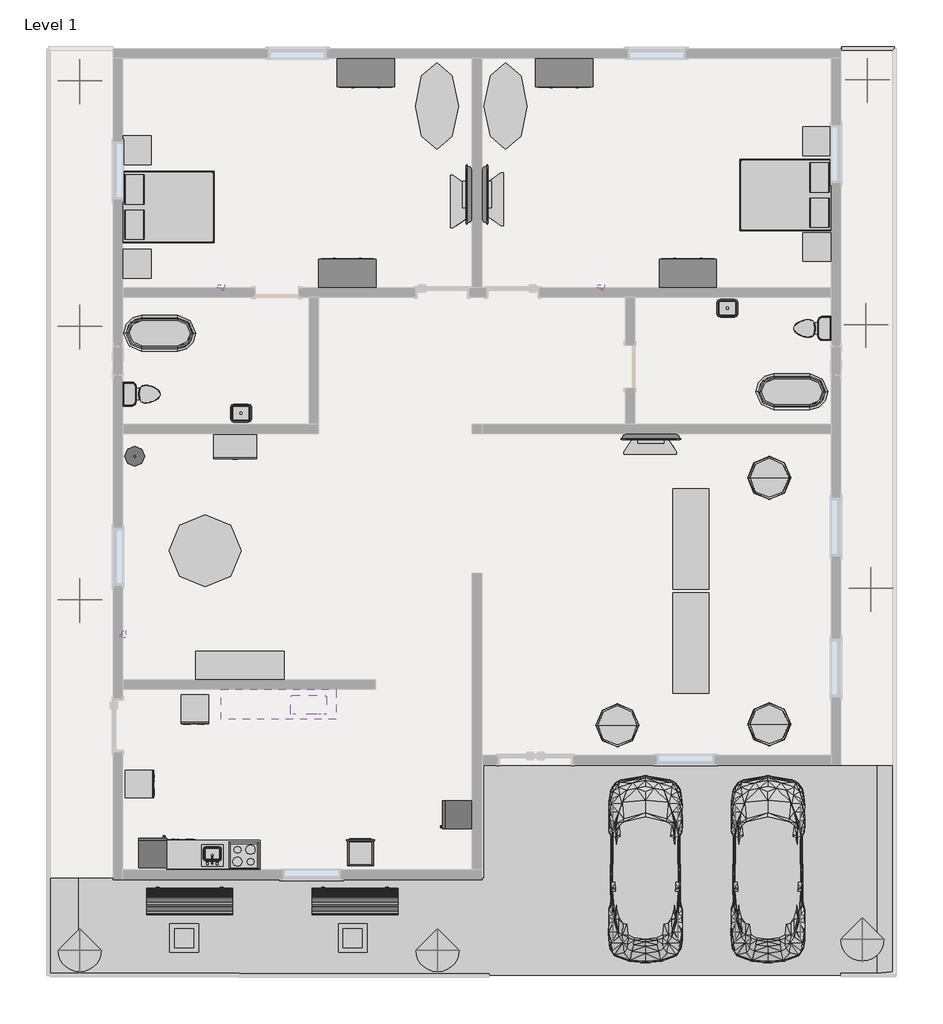
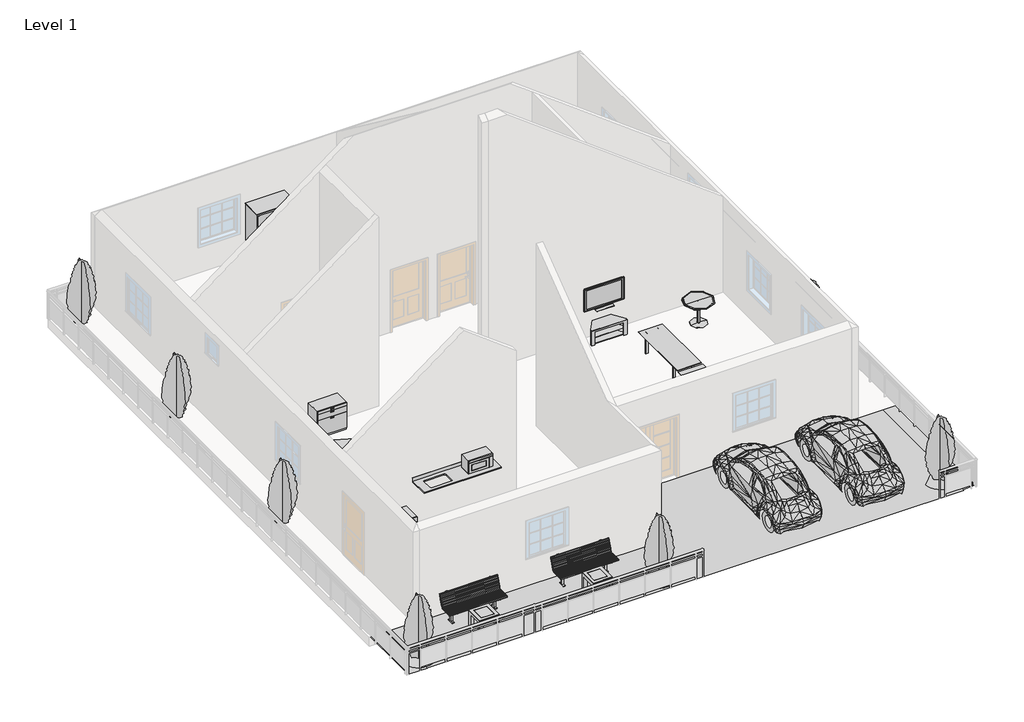
# One storey, part 3 of 3: 30 furniture elements, 17 proxies, 11 geographic elements, 8 flow terminals, 1 railing.
"""IFC4 building model written with IfcOpenShell, lengths in millimetres."""

from ifc_helpers import new_model, si_unit, point, frame, origin, origin_with_axes, place, context, project, spatial, polyline, ellipse_curve, trimmed, outline, extrude, triangles, transform, mapped, element, save
from ifc_brep_helpers import plane_surface, extruded_surface, advanced_brep
from components import proxy_a6faaae8, proxy_53e5fb40, proxy_45b28599, kitchenette_medium_kitchenette_medium_844211aa, proxy_8a8d5ab2, proxy_8b8c2dc4, rpc_beetle_rpc_beetle_3ce7ba48, rpc_picture_frame_rpc_picture_frame_c25e3fe9, proxy_c523a7b7, proxy_66164f77, flow_terminal_871c2e40, flow_terminal_d49f872f, flow_terminal_62a433f7, toilet_domestic_3d_toilet_domestic_3d_f7549cf7, toilet_domestic_3d_toilet_domestic_3d_183bbd19, flow_terminal_b374fae2, furniture_1d2926bd, furniture_c6510c7c, counter_top_w_sink_hole_counter_top_w_sink_hole_22cae41e, furniture_7b927048, furniture_9fa109b2, furniture_e1dba61b, furniture_fdf74506, tv_stand_tv_stand_6ce107e5, furniture_b5c51a22, furniture_92191dda, furniture_bbcc68ce, furniture_027a2ad9, furniture_5bc9ed15, furniture_c80d6d9c, geographic_element_235d1464, rpc_tree_conifer_chinese_juniper_7_1b9786cd

model = new_model("IFC4")

# Units and contexts
model_context = context("Model", 3, world=origin())
ifc_project = project(units=[si_unit("LENGTHUNIT", "METRE", prefix="MILLI")], contexts=[model_context])

# Site, building, storey
site = spatial("IfcSite", under=ifc_project)
building = spatial("IfcBuilding", under=site)
storey = spatial("IfcBuildingStorey", under=building, Name="Level 1", Elevation=0.0)

# Proxies
placement = place(None, origin())
element("IfcBuildingElementProxy", 1, Name="Building Element Proxy", at=placement, inside=storey, context=model_context, shape_type="Tessellation", body=[
    triangles([(-17842.0888458, 13557.9549957, 0.0), (-17105.9465698, 13557.9549957, 0.0), (-17842.0888458, -6127.0451981, 0.0), (-17080.0888458, -4095.0451012, 0.0), (-9244.1892334, -4095.0451012, 0.0), (-9244.1892334, -1656.6451012, 0.0), (-849.4892818, -1762.0254421, 0.0), (-849.4892818, -6127.0451981, 0.0), (-1611.4892818, 13557.9549957, 0.0), (-849.4892818, 13557.9549957, 0.0)], [[3, 4, 1], [6, 4, 5], [4, 2, 1], [2, 4, 6], [2, 6, 9], [7, 6, 5], [4, 3, 5], [5, 8, 7], [8, 5, 3], [9, 7, 10], [9, 6, 7]], closed=False),
])
element("IfcBuildingElementProxy", 2, Name="Building Element Proxy", at=placement, inside=storey, context=model_context, shape_type="Tessellation", body=[
    triangles([(-17817.3124512, -6127.0451981, 0.0), (-18419.3594238, -6127.0451981, 0.0), (-17816.6892334, 13557.9549957, 0.0), (-18438.989621, 13548.4299957, 0.0)], [[4, 2, 1], [1, 3, 4]], closed=False),
])
element("IfcBuildingElementProxy", 3, Name="Building Element Proxy", at=placement, inside=storey, context=model_context, shape_type="Tessellation", body=[
    triangles([(-851.4358927, -6086.4848831, 0.0), (-443.0892697, -6044.4950043, 0.0), (-490.7142697, 13573.8296082, 0.0), (-849.4892818, 13557.9549957, 0.0)], [[4, 1, 2], [2, 3, 4]], closed=False),
])
proxy_shape = proxy_a6faaae8(model_context)
element("IfcBuildingElementProxy", 4, Name="Cook Top-4 Unit2 : 22\" x 20\"", ObjectType="Cook Top-4 Unit2 : 22\" x 20\"", at=placement, inside=storey, context=model_context, shape_type="MappedRepresentation", body=[
    mapped(proxy_shape, transform((-14298.7892853, -3587.0450825, 0.0), x_axis=(-1.0000000000000004, 0.0, 0.0), y_axis=(0.0, -1.0000000000000004, 0.0), z_axis=(0.0, 0.0, 1.0))),
])
proxy_2_shape = proxy_53e5fb40(model_context)
element("IfcBuildingElementProxy", 5, Name="Dishwasher : 23\" x 23 11/16\" x 33 1/2\"", ObjectType="Dishwasher : 23\" x 23 11/16\" x 33 1/2\"", at=placement, inside=storey, context=model_context, shape_type="MappedRepresentation", body=[
    mapped(proxy_2_shape, transform((-16265.9718168, -2439.5330177, 0.0), x_axis=(0.0, 1.0000000000000009, 0.0), y_axis=(-1.0000000000000009, 0.0, 0.0), z_axis=(0.0, 0.0, 1.0))),
])
element("IfcBuildingElementProxy", 6, Name="Dishwasher : 23\" x 23 11/16\" x 33 1/2\"", ObjectType="Dishwasher : 23\" x 23 11/16\" x 33 1/2\"", at=placement, inside=storey, context=model_context, shape_type="MappedRepresentation", body=[
    mapped(proxy_2_shape, transform((-15711.1242223, -733.806712, 0.0), x_axis=(1.0000000000000002, 0.0, 0.0), y_axis=(0.0, 1.0000000000000002, 0.0), z_axis=(0.0, 0.0, 1.0))),
])
proxy_3_shape = proxy_45b28599(model_context)
element("IfcBuildingElementProxy", 7, Name="Dishwasher : 24\" x 24\" x 34\"", ObjectType="Dishwasher : 24\" x 24\" x 34\"", at=placement, inside=storey, context=model_context, shape_type="MappedRepresentation", body=[
    mapped(proxy_3_shape, transform((-15249.9718168, -3295.1955177, 0.0), x_axis=(-1.0000000000000004, 0.0, 0.0), y_axis=(0.0, -1.0000000000000004, 0.0), z_axis=(0.0, 0.0, 1.0))),
])
kitchenette_medium_kitchenette_medium_shape = kitchenette_medium_kitchenette_medium_844211aa(model_context)
element("IfcBuildingElementProxy", 8, Name="Kitchenette - Medium : Kitchenette - Medium", ObjectType="Kitchenette - Medium : Kitchenette - Medium", at=placement, inside=storey, context=model_context, shape_type="MappedRepresentation", body=[
    mapped(kitchenette_medium_kitchenette_medium_shape, transform((-14622.9515804, -3891.8450825, 0.0), x_axis=(-1.0000000000000004, 0.0, 0.0), y_axis=(0.0, -1.0000000000000004, 0.0), z_axis=(0.0, 0.0, 1.0))),
])
proxy_4_shape = proxy_8a8d5ab2(model_context)
element("IfcBuildingElementProxy", 9, Name="Microwave : 30\" x 16\" x 18\"", ObjectType="Microwave : 30\" x 16\" x 18\"", at=placement, inside=storey, context=model_context, shape_type="MappedRepresentation", body=[
    mapped(proxy_4_shape, transform((-13427.4821626, -27.2145766, 609.6), x_axis=(1.0, 0.0, 0.0), y_axis=(0.0, 1.0, 0.0), z_axis=(0.0, 0.0, 1.0))),
])
proxy_5_shape = proxy_8b8c2dc4(model_context)
element("IfcBuildingElementProxy", 10, Name="Oven Double-Built-in : 21 1/2\" x 39 1/4\" x 21\"", ObjectType="Oven Double-Built-in : 21 1/2\" x 39 1/4\" x 21\"", at=placement, inside=storey, context=model_context, shape_type="MappedRepresentation", body=[
    mapped(proxy_5_shape, transform((-11857.4642126, -3395.1792235, 0.0), x_axis=(-1.0000000000000013, 0.0, 0.0), y_axis=(0.0, -1.0000000000000013, 0.0), z_axis=(0.0, 0.0, 1.0))),
])
rpc_beetle_rpc_beetle_shape = rpc_beetle_rpc_beetle_3ce7ba48(model_context)
element("IfcBuildingElementProxy", 11, Name="RPC Beetle : RPC Beetle", ObjectType="RPC Beetle : RPC Beetle", at=placement, inside=storey, context=model_context, shape_type="MappedRepresentation", body=[
    mapped(rpc_beetle_rpc_beetle_shape, transform((-3160.8892853, -5111.0450825, 0.0), x_axis=(1.0, 0.0, 0.0), y_axis=(0.0, 1.0, 0.0), z_axis=(0.0, 0.0, 1.0))),
])
element("IfcBuildingElementProxy", 12, Name="RPC Beetle : RPC Beetle", ObjectType="RPC Beetle : RPC Beetle", at=placement, inside=storey, context=model_context, shape_type="MappedRepresentation", body=[
    mapped(rpc_beetle_rpc_beetle_shape, transform((-5764.3892853, -5111.0450825, 0.0), x_axis=(1.0, 0.0, 0.0), y_axis=(0.0, 1.0, 0.0), z_axis=(0.0, 0.0, 1.0))),
])
rpc_picture_frame_rpc_picture_frame_shape = rpc_picture_frame_rpc_picture_frame_c25e3fe9(model_context)
element("IfcBuildingElementProxy", 13, Name="RPC Picture Frame : RPC Picture Frame", ObjectType="RPC Picture Frame : RPC Picture Frame", at=placement, inside=storey, context=model_context, shape_type="MappedRepresentation", body=[
    mapped(rpc_picture_frame_rpc_picture_frame_shape, transform((-14782.9146553, 8477.9549175, 2133.6), x_axis=(-1.0000000000000004, 0.0, 0.0), y_axis=(0.0, -1.0000000000000004, 0.0), z_axis=(0.0, 0.0, 1.0))),
])
element("IfcBuildingElementProxy", 14, Name="RPC Picture Frame : RPC Picture Frame", ObjectType="RPC Picture Frame : RPC Picture Frame", at=placement, inside=storey, context=model_context, shape_type="MappedRepresentation", body=[
    mapped(rpc_picture_frame_rpc_picture_frame_shape, transform((-6713.5023261, 8477.9549175, 2133.6), x_axis=(-1.0, 0.0, 0.0), y_axis=(0.0, -1.0, 0.0), z_axis=(0.0, 0.0, 1.0))),
])
element("IfcBuildingElementProxy", 15, Name="RPC Picture Frame : RPC Picture Frame", ObjectType="RPC Picture Frame : RPC Picture Frame", at=placement, inside=storey, context=model_context, shape_type="MappedRepresentation", body=[
    mapped(rpc_picture_frame_rpc_picture_frame_shape, transform((-16876.8892853, 1119.0822446, 2133.6), x_axis=(0.0, 1.0000000000000004, 0.0), y_axis=(-1.0000000000000004, 0.0, 0.0), z_axis=(0.0, 0.0, 1.0))),
])
proxy_6_shape = proxy_c523a7b7(model_context)
element("IfcBuildingElementProxy", 16, Name="Refrigerator : 24\" x 25\" LH", ObjectType="Refrigerator : 24\" x 25\" LH", at=placement, inside=storey, context=model_context, shape_type="MappedRepresentation", body=[
    mapped(proxy_6_shape, transform((-16235.5392853, -3541.396111, 0.0), x_axis=(-1.0000000000000004, 0.0, 0.0), y_axis=(0.0, -1.0000000000000004, 0.0), z_axis=(0.0, 0.0, 1.0))),
])
proxy_7_shape = proxy_66164f77(model_context)
element("IfcBuildingElementProxy", 17, Name="Refrigerator : 24\" x 25\" RH", ObjectType="Refrigerator : 24\" x 25\" RH", at=placement, inside=storey, context=model_context, shape_type="MappedRepresentation", body=[
    mapped(proxy_7_shape, transform((-9745.8392853, -2718.2940539, 0.0), x_axis=(0.0, -1.0000000000000007, 0.0), y_axis=(1.0000000000000007, 0.0, 0.0), z_axis=(0.0, 0.0, 1.0))),
])

# Flow terminals
flow_terminal_shape = flow_terminal_871c2e40(model_context)
element("IfcFlowTerminal", 18, ObjectType="Sink Kitchen-Island : 18\" x 18\"", at=placement, inside=storey, context=model_context, shape_type="MappedRepresentation", body=[
    mapped(flow_terminal_shape, transform((-14956.2000447, -3584.6996813, -14.4), x_axis=(-1.0000000000000004, 0.0, 0.0), y_axis=(0.0, -1.0000000000000004, 0.0), z_axis=(0.0, 0.0, 1.0))),
])
flow_terminal_2_shape = flow_terminal_d49f872f(model_context)
element("IfcFlowTerminal", 19, ObjectType="Sink Vanity-Round : 19\" x 19\"", at=placement, inside=storey, context=model_context, shape_type="MappedRepresentation", body=[
    mapped(flow_terminal_2_shape, transform((-16533.4036272, 4799.903177, 609.6), x_axis=(0.0, 1.0, 0.0), y_axis=(-1.0, 0.0, 0.0), z_axis=(0.0, 0.0, 1.0))),
])
flow_terminal_3_shape = flow_terminal_62a433f7(model_context)
element("IfcFlowTerminal", 20, ObjectType="Sink Vanity-Square : 20\" x 18\"", at=placement, inside=storey, context=model_context, shape_type="MappedRepresentation", body=[
    mapped(flow_terminal_3_shape, transform((-14346.6000447, 5762.5003187, 609.6), x_axis=(-1.0000000000000004, 0.0, 0.0), y_axis=(0.0, -1.0000000000000004, 0.0), z_axis=(0.0, 0.0, 1.0))),
])
element("IfcFlowTerminal", 21, ObjectType="Sink Vanity-Square : 20\" x 18\"", at=placement, inside=storey, context=model_context, shape_type="MappedRepresentation", body=[
    mapped(flow_terminal_3_shape, transform((-4040.1785259, 8094.6095164, 609.6), x_axis=(1.0, 0.0, 0.0), y_axis=(0.0, 1.0, 0.0), z_axis=(0.0, 0.0, 1.0))),
])
toilet_domestic_3d_toilet_domestic_3d_shape = toilet_domestic_3d_toilet_domestic_3d_f7549cf7(model_context)
toilet_domestic_3d_toilet_domestic_3d_2_shape = toilet_domestic_3d_toilet_domestic_3d_183bbd19(model_context)
element("IfcFlowTerminal", 22, ObjectType="Toilet-Domestic-3D : Toilet-Domestic-3D", at=placement, inside=storey, context=model_context, shape_type="MappedRepresentation", body=[
    mapped(toilet_domestic_3d_toilet_domestic_3d_shape, transform((-2309.3853126, 7614.3549175, 0.0), x_axis=(0.0, -1.0, 0.0), y_axis=(1.0, 0.0, 0.0), z_axis=(0.0, 0.0, 1.0))),
    mapped(toilet_domestic_3d_toilet_domestic_3d_2_shape, transform((-2309.3853126, 7614.3549175, 0.0), x_axis=(0.0, -1.0, 0.0), y_axis=(1.0, 0.0, 0.0), z_axis=(0.0, 0.0, 1.0))),
])
element("IfcFlowTerminal", 23, ObjectType="Toilet-Domestic-3D : Toilet-Domestic-3D", at=placement, inside=storey, context=model_context, shape_type="MappedRepresentation", body=[
    mapped(toilet_domestic_3d_toilet_domestic_3d_shape, transform((-16382.1932579, 6217.3549175, 0.0), x_axis=(0.0, 1.0000000000000002, 0.0), y_axis=(-1.0000000000000002, 0.0, 0.0), z_axis=(0.0, 0.0, 1.0))),
    mapped(toilet_domestic_3d_toilet_domestic_3d_2_shape, transform((-16382.1932579, 6217.3549175, 0.0), x_axis=(0.0, 1.0000000000000002, 0.0), y_axis=(-1.0000000000000002, 0.0, 0.0), z_axis=(0.0, 0.0, 1.0))),
])
flow_terminal_4_shape = flow_terminal_b374fae2(model_context)
element("IfcFlowTerminal", 24, ObjectType="Tub-Free Standing-3D : 30\" x 60\"", at=placement, inside=storey, context=model_context, shape_type="MappedRepresentation", body=[
    mapped(flow_terminal_4_shape, transform((-16089.4892853, 7512.7549175, 0.0), x_axis=(0.0, 1.0000000000000002, 0.0), y_axis=(-1.0000000000000002, 0.0, 0.0), z_axis=(0.0, 0.0, 1.0))),
])
element("IfcFlowTerminal", 25, ObjectType="Tub-Free Standing-3D : 30\" x 60\"", at=placement, inside=storey, context=model_context, shape_type="MappedRepresentation", body=[
    mapped(flow_terminal_4_shape, transform((-2652.8892853, 6268.1549175, 0.0), x_axis=(0.0, -1.0000000000000009, 0.0), y_axis=(1.0000000000000009, 0.0, 0.0), z_axis=(0.0, 0.0, 1.0))),
])

# Furniture
furniture_shape = furniture_1d2926bd(model_context)
element("IfcFurniture", 26, ObjectType="Bed-Box : Queen 60\" x 79\"", at=placement, inside=storey, context=model_context, shape_type="MappedRepresentation", body=[
    mapped(furniture_shape, transform((-16171.5187935, 9853.3024585, 0.0), x_axis=(0.0, 1.0000000000000002, 0.0), y_axis=(-1.0000000000000002, 0.0, 0.0), z_axis=(0.0, 0.0, 1.0))),
])
element("IfcFurniture", 27, ObjectType="Bed-Box : Queen 60\" x 79\"", at=placement, inside=storey, context=model_context, shape_type="MappedRepresentation", body=[
    mapped(furniture_shape, transform((-2520.0597771, 10785.6073766, 0.0), x_axis=(0.0, -1.0000000000000004, 0.0), y_axis=(1.0000000000000004, 0.0, 0.0), z_axis=(0.0, 0.0, 1.0))),
])
furniture_2_shape = furniture_c6510c7c(model_context)
element("IfcFurniture", 28, ObjectType="Counter Top w Sink Hole : 24\" Depth", at=placement, inside=storey, context=model_context, shape_type="MappedRepresentation", body=[
    mapped(furniture_2_shape, transform((-15156.3515804, -3891.8450825, -14.4), x_axis=(-1.0000000000000004, 0.0, 0.0), y_axis=(0.0, -1.0000000000000004, 0.0), z_axis=(0.0, 0.0, 1.0))),
])
counter_top_w_sink_hole_counter_top_w_sink_hole_shape = counter_top_w_sink_hole_counter_top_w_sink_hole_22cae41e(model_context)
element("IfcFurniture", 29, ObjectType="Counter Top w Sink Hole : Counter Top w Sink Hole", at=placement, inside=storey, context=model_context, shape_type="MappedRepresentation", body=[
    mapped(counter_top_w_sink_hole_counter_top_w_sink_hole_shape, transform((-13580.9269902, -56.4450825, 609.6), x_axis=(1.0, 0.0, 0.0), y_axis=(0.0, 1.0, 0.0), z_axis=(0.0, 0.0, 1.0))),
])
furniture_3_shape = furniture_7b927048(model_context)
element("IfcFurniture", 30, ObjectType="Credenza : 72\" x 24\"", at=placement, inside=storey, context=model_context, shape_type="MappedRepresentation", body=[
    mapped(furniture_3_shape, transform((-14447.2335476, 446.9745897, 0.0), x_axis=(1.0, 0.0, 0.0), y_axis=(0.0, 1.0, 0.0), z_axis=(0.0, 0.0, 1.0))),
])
furniture_4_shape = furniture_9fa109b2(model_context)
element("IfcFurniture", 31, ObjectType="Dresser : 48\" x 72\" x 24\"", at=placement, inside=storey, context=model_context, shape_type="MappedRepresentation", body=[
    mapped(furniture_4_shape, transform((-12370.8825451, 8419.5919634, 0.0), x_axis=(-1.0000000000000004, 0.0, 0.0), y_axis=(0.0, -1.0000000000000004, 0.0), z_axis=(0.0, 0.0, 1.0))),
])
element("IfcFurniture", 32, ObjectType="Dresser : 48\" x 72\" x 24\"", at=placement, inside=storey, context=model_context, shape_type="MappedRepresentation", body=[
    mapped(furniture_4_shape, transform((-11438.7960255, 13413.1178716, 0.0), x_axis=(1.0, 0.0, 0.0), y_axis=(0.0, 1.0, 0.0), z_axis=(0.0, 0.0, 1.0))),
])
element("IfcFurniture", 33, ObjectType="Dresser : 48\" x 72\" x 24\"", at=placement, inside=storey, context=model_context, shape_type="MappedRepresentation", body=[
    mapped(furniture_4_shape, transform((-7222.3960255, 13413.1178716, 0.0), x_axis=(1.0, 0.0, 0.0), y_axis=(0.0, 1.0, 0.0), z_axis=(0.0, 0.0, 1.0))),
])
element("IfcFurniture", 34, ObjectType="Dresser : 48\" x 72\" x 24\"", at=placement, inside=storey, context=model_context, shape_type="MappedRepresentation", body=[
    mapped(furniture_4_shape, transform((-5131.8825451, 8419.5919634, 0.0), x_axis=(-1.0000000000000004, 0.0, 0.0), y_axis=(0.0, -1.0000000000000004, 0.0), z_axis=(0.0, 0.0, 1.0))),
])
furniture_5_shape = furniture_e1dba61b(model_context)
element("IfcFurniture", 35, ObjectType="Storage Pedestal : 20\" x 36\" x 36\"", at=placement, inside=storey, context=model_context, shape_type="MappedRepresentation", body=[
    mapped(furniture_5_shape, transform((-14309.2667714, 6034.0732936, 0.0), x_axis=(1.0, 0.0, 0.0), y_axis=(0.0, 1.0, 0.0), z_axis=(0.0, 0.0, 1.0))),
])
furniture_6_shape = furniture_fdf74506(model_context)
element("IfcFurniture", 36, ObjectType="TV - Flat Screen : 50\"", at=placement, inside=storey, context=model_context, shape_type="MappedRepresentation", body=[
    mapped(furniture_6_shape, transform((-9505.9279089, 10455.2104034, 914.4), x_axis=(0.0, -1.0000000000000004, 0.0), y_axis=(1.0000000000000004, 0.0, 0.0), z_axis=(0.0, 0.0, 1.0))),
])
element("IfcFurniture", 37, ObjectType="TV - Flat Screen : 50\"", at=placement, inside=storey, context=model_context, shape_type="MappedRepresentation", body=[
    mapped(furniture_6_shape, transform((-9185.6506616, 10463.0994317, 914.4), x_axis=(0.0, 1.0000000000000002, 0.0), y_axis=(-1.0000000000000002, 0.0, 0.0), z_axis=(0.0, 0.0, 1.0))),
])
element("IfcFurniture", 38, ObjectType="TV - Flat Screen : 50\"", at=placement, inside=storey, context=model_context, shape_type="MappedRepresentation", body=[
    mapped(furniture_6_shape, transform((-5646.1447711, 5320.6162939, 914.4), x_axis=(1.0, 0.0, 0.0), y_axis=(0.0, 1.0, 0.0), z_axis=(0.0, 0.0, 1.0))),
])
tv_stand_tv_stand_shape = tv_stand_tv_stand_6ce107e5(model_context)
element("IfcFurniture", 39, ObjectType="TV Stand : TV Stand", at=placement, inside=storey, context=model_context, shape_type="MappedRepresentation", body=[
    mapped(tv_stand_tv_stand_shape, transform((-9447.3892853, 10431.9429196, 0.0), x_axis=(0.0, -1.0, 0.0), y_axis=(1.0, 0.0, 0.0), z_axis=(0.0, 0.0, 1.0))),
])
element("IfcFurniture", 40, ObjectType="TV Stand : TV Stand", at=placement, inside=storey, context=model_context, shape_type="MappedRepresentation", body=[
    mapped(tv_stand_tv_stand_shape, transform((-9244.1892853, 10232.3669155, 0.0), x_axis=(0.0, 1.0, 0.0), y_axis=(-1.0, 0.0, 0.0), z_axis=(0.0, 0.0, 1.0))),
])
element("IfcFurniture", 41, ObjectType="TV Stand : TV Stand", at=placement, inside=storey, context=model_context, shape_type="MappedRepresentation", body=[
    mapped(tv_stand_tv_stand_shape, transform((-5787.4891902, 5402.9061632, 0.0), x_axis=(1.0000000000000007, 0.0, 0.0), y_axis=(0.0, 1.0000000000000007, 0.0), z_axis=(0.0, 0.0, 1.0))),
])
furniture_7_shape = furniture_b5c51a22(model_context)
element("IfcFurniture", 42, ObjectType="Table-Coffee : 24\" x 24\" x 24\"", at=placement, inside=storey, context=model_context, shape_type="MappedRepresentation", body=[
    mapped(furniture_7_shape, transform((-15587.055052, -5434.8561603, 0.0), x_axis=(1.0, 0.0, 0.0), y_axis=(0.0, 1.0, 0.0), z_axis=(0.0, 0.0, 1.0))),
])
element("IfcFurniture", 43, ObjectType="Table-Coffee : 24\" x 24\" x 24\"", at=placement, inside=storey, context=model_context, shape_type="MappedRepresentation", body=[
    mapped(furniture_7_shape, transform((-12005.655052, -5434.8561603, 0.0), x_axis=(1.0, 0.0, 0.0), y_axis=(0.0, 1.0, 0.0), z_axis=(0.0, 0.0, 1.0))),
])
furniture_8_shape = furniture_92191dda(model_context)
element("IfcFurniture", 44, ObjectType="Table-Dining : 30\" x 84\" x 22\"", at=placement, inside=storey, context=model_context, shape_type="MappedRepresentation", body=[
    mapped(furniture_8_shape, transform((-4703.9782075, 915.8891509, 0.0), x_axis=(0.0, 1.0, 0.0), y_axis=(-1.0, 0.0, 0.0), z_axis=(0.0, 0.0, 1.0))),
])
element("IfcFurniture", 45, ObjectType="Table-Dining : 30\" x 84\" x 22\"", at=placement, inside=storey, context=model_context, shape_type="MappedRepresentation", body=[
    mapped(furniture_8_shape, transform((-4703.9782075, 3125.6891509, 0.0), x_axis=(0.0, 1.0, 0.0), y_axis=(-1.0, 0.0, 0.0), z_axis=(0.0, 0.0, 1.0))),
])
furniture_9_shape = furniture_bbcc68ce(model_context)
element("IfcFurniture", 46, ObjectType="Table-Dining Round w Chairs : 60\" Diameter", at=placement, inside=storey, context=model_context, shape_type="MappedRepresentation", body=[
    mapped(furniture_9_shape, transform((-15227.9712525, 3074.8336061, 0.0), x_axis=(1.0, 0.0, 0.0), y_axis=(0.0, 1.0, 0.0), z_axis=(0.0, 0.0, 1.0))),
])
furniture_10_shape = furniture_027a2ad9(model_context)
element("IfcFurniture", 47, ObjectType="Table-Ellipse : 72\" x 36\"", at=placement, inside=storey, context=model_context, shape_type="MappedRepresentation", body=[
    mapped(furniture_10_shape, transform((-8736.1892853, 12338.7549175, 0.0), x_axis=(0.0, 1.0000000000000002, 0.0), y_axis=(-1.0000000000000002, 0.0, 0.0), z_axis=(0.0, 0.0, 1.0))),
])
element("IfcFurniture", 48, ObjectType="Table-Ellipse : 72\" x 36\"", at=placement, inside=storey, context=model_context, shape_type="MappedRepresentation", body=[
    mapped(furniture_10_shape, transform((-10196.6892853, 12338.7549175, 0.0), x_axis=(0.0, 1.0000000000000002, 0.0), y_axis=(-1.0000000000000002, 0.0, 0.0), z_axis=(0.0, 0.0, 1.0))),
])
furniture_11_shape = furniture_5bc9ed15(model_context)
element("IfcFurniture", 49, ObjectType="Table-Night Stand : 24\" x 24\" x 30\"", at=placement, inside=storey, context=model_context, shape_type="MappedRepresentation", body=[
    mapped(furniture_11_shape, transform((-16880.6229156, 8681.1549175, 0.0), x_axis=(1.0, 0.0, 0.0), y_axis=(0.0, 1.0, 0.0), z_axis=(0.0, 0.0, 1.0))),
])
element("IfcFurniture", 50, ObjectType="Table-Night Stand : 24\" x 24\" x 30\"", at=placement, inside=storey, context=model_context, shape_type="MappedRepresentation", body=[
    mapped(furniture_11_shape, transform((-16880.6229156, 11094.1549175, 0.0), x_axis=(1.0, 0.0, 0.0), y_axis=(0.0, 1.0, 0.0), z_axis=(0.0, 0.0, 1.0))),
])
element("IfcFurniture", 51, ObjectType="Table-Night Stand : 24\" x 24\" x 30\"", at=placement, inside=storey, context=model_context, shape_type="MappedRepresentation", body=[
    mapped(furniture_11_shape, transform((-2428.0229156, 9036.7549175, 0.0), x_axis=(1.0, 0.0, 0.0), y_axis=(0.0, 1.0, 0.0), z_axis=(0.0, 0.0, 1.0))),
])
element("IfcFurniture", 52, ObjectType="Table-Night Stand : 24\" x 24\" x 30\"", at=placement, inside=storey, context=model_context, shape_type="MappedRepresentation", body=[
    mapped(furniture_11_shape, transform((-2428.0229156, 11284.6549175, 0.0), x_axis=(1.0, 0.0, 0.0), y_axis=(0.0, 1.0, 0.0), z_axis=(0.0, 0.0, 1.0))),
])
furniture_12_shape = furniture_c80d6d9c(model_context)
element("IfcFurniture", 53, ObjectType="Table-Round : 36\" Diameter", at=placement, inside=storey, context=model_context, shape_type="MappedRepresentation", body=[
    mapped(furniture_12_shape, transform((-3135.4892853, -799.3950825, 0.0), x_axis=(1.0, 0.0, 0.0), y_axis=(0.0, 1.0, 0.0), z_axis=(0.0, 0.0, 1.0))),
])
element("IfcFurniture", 54, ObjectType="Table-Round : 36\" Diameter", at=placement, inside=storey, context=model_context, shape_type="MappedRepresentation", body=[
    mapped(furniture_12_shape, transform((-6361.2892853, -818.4450825, 0.0), x_axis=(1.0, 0.0, 0.0), y_axis=(0.0, 1.0, 0.0), z_axis=(0.0, 0.0, 1.0))),
])
element("IfcFurniture", 55, ObjectType="Table-Round : 36\" Diameter", at=placement, inside=storey, context=model_context, shape_type="MappedRepresentation", body=[
    mapped(furniture_12_shape, transform((-3135.4892853, 4439.3549175, 0.0), x_axis=(1.0, 0.0, 0.0), y_axis=(0.0, 1.0, 0.0), z_axis=(0.0, 0.0, 1.0))),
])

# Geographic elements
geographic_element_shape = geographic_element_235d1464(model_context)
element("IfcGeographicElement", 56, ObjectType="Park Bench : 72\"", at=placement, inside=storey, context=model_context, shape_type="MappedRepresentation", body=[
    mapped(geographic_element_shape, transform((-11936.5892853, -4526.8450825, 0.0), x_axis=(1.0, 0.0, 0.0), y_axis=(0.0, 1.0, 0.0), z_axis=(0.0, 0.0, 1.0))),
])
element("IfcGeographicElement", 57, ObjectType="Park Bench : 72\"", at=placement, inside=storey, context=model_context, shape_type="MappedRepresentation", body=[
    mapped(geographic_element_shape, transform((-15454.4892853, -4526.8450825, 0.0), x_axis=(1.0, 0.0, 0.0), y_axis=(0.0, 1.0, 0.0), z_axis=(0.0, 0.0, 1.0))),
])
rpc_tree_conifer_chinese_juniper_7_shape = rpc_tree_conifer_chinese_juniper_7_1b9786cd(model_context)
element("IfcGeographicElement", 58, ObjectType="RPC Tree - Conifer : Chinese Juniper - 7'", at=placement, inside=storey, context=model_context, shape_type="MappedRepresentation", body=[
    mapped(rpc_tree_conifer_chinese_juniper_7_shape, transform((-1154.4859564, -5365.0450825, 0.0), x_axis=(1.0, 0.0, 0.0), y_axis=(0.0, 1.0, 0.0), z_axis=(0.0, 0.0, 1.0))),
])
element("IfcGeographicElement", 59, ObjectType="RPC Tree - Conifer : Chinese Juniper - 7'", at=placement, inside=storey, context=model_context, shape_type="MappedRepresentation", body=[
    mapped(rpc_tree_conifer_chinese_juniper_7_shape, transform((-10184.1859564, -5593.6450825, 0.0), x_axis=(1.0, 0.0, 0.0), y_axis=(0.0, 1.0, 0.0), z_axis=(0.0, 0.0, 1.0))),
])
element("IfcGeographicElement", 60, ObjectType="RPC Tree - Conifer : Chinese Juniper - 7'", at=placement, inside=storey, context=model_context, shape_type="MappedRepresentation", body=[
    mapped(rpc_tree_conifer_chinese_juniper_7_shape, transform((-17791.4859564, -5593.6450825, 0.0), x_axis=(1.0, 0.0, 0.0), y_axis=(0.0, 1.0, 0.0), z_axis=(0.0, 0.0, 1.0))),
])
element("IfcGeographicElement", 61, ObjectType="RPC Tree - Conifer : Chinese Juniper - 7'", at=placement, inside=storey, context=model_context, shape_type="MappedRepresentation", body=[
    mapped(rpc_tree_conifer_chinese_juniper_7_shape, transform((-17791.4859564, 1848.5549175, 0.0), x_axis=(1.0, 0.0, 0.0), y_axis=(0.0, 1.0, 0.0), z_axis=(0.0, 0.0, 1.0))),
])
element("IfcGeographicElement", 62, ObjectType="RPC Tree - Conifer : Chinese Juniper - 7'", at=placement, inside=storey, context=model_context, shape_type="MappedRepresentation", body=[
    mapped(rpc_tree_conifer_chinese_juniper_7_shape, transform((-17791.4859564, 7665.1549175, 0.0), x_axis=(1.0, 0.0, 0.0), y_axis=(0.0, 1.0, 0.0), z_axis=(0.0, 0.0, 1.0))),
])
element("IfcGeographicElement", 63, ObjectType="RPC Tree - Conifer : Chinese Juniper - 7'", at=placement, inside=storey, context=model_context, shape_type="MappedRepresentation", body=[
    mapped(rpc_tree_conifer_chinese_juniper_7_shape, transform((-17791.4859564, 12872.1549175, 0.0), x_axis=(1.0, 0.0, 0.0), y_axis=(0.0, 1.0, 0.0), z_axis=(0.0, 0.0, 1.0))),
])
element("IfcGeographicElement", 64, ObjectType="RPC Tree - Conifer : Chinese Juniper - 7'", at=placement, inside=storey, context=model_context, shape_type="MappedRepresentation", body=[
    mapped(rpc_tree_conifer_chinese_juniper_7_shape, transform((-1052.8859564, 12897.5549175, 0.0), x_axis=(1.0, 0.0, 0.0), y_axis=(0.0, 1.0, 0.0), z_axis=(0.0, 0.0, 1.0))),
])
element("IfcGeographicElement", 65, ObjectType="RPC Tree - Conifer : Chinese Juniper - 7'", at=placement, inside=storey, context=model_context, shape_type="MappedRepresentation", body=[
    mapped(rpc_tree_conifer_chinese_juniper_7_shape, transform((-1078.2859564, 7690.5549175, 0.0), x_axis=(1.0, 0.0, 0.0), y_axis=(0.0, 1.0, 0.0), z_axis=(0.0, 0.0, 1.0))),
])
element("IfcGeographicElement", 66, ObjectType="RPC Tree - Conifer : Chinese Juniper - 7'", at=placement, inside=storey, context=model_context, shape_type="MappedRepresentation", body=[
    mapped(rpc_tree_conifer_chinese_juniper_7_shape, transform((-976.6859564, 2089.8549175, 0.0), x_axis=(1.0, 0.0, 0.0), y_axis=(0.0, 1.0, 0.0), z_axis=(0.0, 0.0, 1.0))),
])

# Railing
element("IfcRailing", 67, ObjectType="Glass Panel - Bottom Fill", at=placement, inside=storey, context=model_context, shape_type="SolidModel", body=[
    advanced_brep(
    [(-478.0142853, 13526.2049175, 914.4), (-478.0142853, 13602.4049175, 914.4), (-1595.6142853, 13526.2049175, 914.4), (-1595.6142853, 13602.4049175, 914.4)],
    [
        (0, 1, ellipse_curve(frame((-478.0142853, 13564.3049175, 914.4), z_axis=(1.0, 0.0, 0.0), x_axis=(0.0, 1.0, 0.0)), 38.1, 28.575)),
        (1, 0, ellipse_curve(frame((-478.0142853, 13564.3049175, 914.4), z_axis=(1.0, 0.0, 0.0), x_axis=(0.0, 1.0, 0.0)), 38.1, 28.575)),
        (2, 3, ellipse_curve(frame((-1595.6142853, 13564.3049175, 914.4), z_axis=(-1.0, 0.0, 0.0), x_axis=(0.0, 1.0, 0.0)), 38.1, 28.575)),
        (3, 2, ellipse_curve(frame((-1595.6142853, 13564.3049175, 914.4), z_axis=(-1.0, 0.0, 0.0), x_axis=(0.0, 1.0, 0.0)), 38.1, 28.575)),
        (0, 2),
        (3, 1),
    ],
    [
        plane_surface(frame((-478.0142853, 13564.3049175, 914.4), z_axis=(1.0, 0.0, 0.0), x_axis=(0.0, -1.0, 0.0))),
        plane_surface(frame((-1595.6142853, 13564.3049175, 914.4), z_axis=(-1.0, 0.0, 0.0), x_axis=(0.0, -1.0, 0.0))),
        extruded_surface(trimmed(ellipse_curve(frame((-1595.6142853, 13564.3049175, 914.4), z_axis=(1.0, 0.0, 0.0), x_axis=(0.0, 1.0, 0.0)), 38.1, 28.575), [point((-1595.6142853, 13526.2049175, 914.4))], [point((-1595.6142853, 13602.4049175, 914.4))], True, "CARTESIAN"), (1117.6, 0.0, 0.0), 1117.6),
        extruded_surface(trimmed(ellipse_curve(frame((-1595.6142853, 13564.3049175, 914.4), z_axis=(1.0, 0.0, 0.0), x_axis=(0.0, 1.0, 0.0)), 38.1, 28.575), [point((-1595.6142853, 13602.4049175, 914.4))], [point((-1595.6142853, 13526.2049175, 914.4))], True, "CARTESIAN"), (1117.6, 0.0, 0.0), 1117.6),
    ],
    [
        (0, [[1, 2]]),
        (1, [[3, 4]]),
        (2, [[-1, 5, -4, 6]]),
        (3, [[-2, -6, -3, -5]]),
    ],
),
    extrude(outline(polyline([(-478.0142853, 13577.0049175), (-478.0142853, 13551.6049175), (-1595.6142853, 13551.6049175), (-1595.6142853, 13577.0049175), (-478.0142853, 13577.0049175)])), frame((0.0, 0.0, 800.1), z_axis=(0.0, 0.0, 1.0), x_axis=(1.0, 0.0, 0.0)), (0.0, 0.0, 1.0), 25.4),
    extrude(outline(polyline([(-478.0142853, 13577.0049175), (-478.0142853, 13551.6049175), (-1595.6142853, 13551.6049175), (-1595.6142853, 13577.0049175), (-478.0142853, 13577.0049175)])), frame((0.0, 0.0, 698.5), z_axis=(0.0, 0.0, 1.0), x_axis=(1.0, 0.0, 0.0)), (0.0, 0.0, 1.0), 25.4),
    extrude(outline(polyline([(-1436.8642853, 13589.7049175), (-1436.8642853, 13538.9049175), (-1449.5642853, 13538.9049175), (-1449.5642853, 13589.7049175), (-1436.8642853, 13589.7049175)])), origin_with_axes(), (0.0, 0.0, 1.0), 885.6788223),
    extrude(outline(polyline([(-630.4142853, 13557.7697605), (-1443.2142853, 13557.7697605), (-1443.2142853, 13564.1197605), (-630.4142853, 13564.1197605), (-630.4142853, 13557.7697605)])), frame((0.0, 0.0, 101.6), z_axis=(0.0, 0.0, 1.0), x_axis=(1.0, 0.0, 0.0)), (0.0, 0.0, 1.0), 596.9),
    extrude(outline(polyline([(-624.0642853, 13589.7049175), (-624.0642853, 13538.9049175), (-636.7642853, 13538.9049175), (-636.7642853, 13589.7049175), (-624.0642853, 13589.7049175)])), origin_with_axes(), (0.0, 0.0, 1.0), 885.6788223),
    extrude(outline(polyline([(-1582.9142853, 13573.8299175), (-1582.9142853, 13554.7799175), (-1601.9642853, 13554.7799175), (-1601.9642853, 13573.8299175), (-1582.9142853, 13573.8299175)])), origin_with_axes(), (0.0, 0.0, 1.0), 885.6788223),
    extrude(outline(polyline([(-471.6642853, 13573.8299175), (-471.6642853, 13554.7799175), (-490.7142853, 13554.7799175), (-490.7142853, 13573.8299175), (-471.6642853, 13573.8299175)])), origin_with_axes(), (0.0, 0.0, 1.0), 885.6788223),
])

save(model, "model.ifc")

# Revit data of these elements
# Type "Cook Top-4 Unit2 : 22\" x 20\""
#   Depth = 1' - 8"
#   Width = 1' - 10"
#   Burner Material = Steel, Chrome Plated
#   Cooktop Material = Steel, Polished
#   Default Elevation = 0
#   Assembly Code = ""
# Type "Dishwasher : 23\" x 23 11/16\" x 33 1/2\""
#   Label = "DW"
#   Assembly Code = "E1090400"
#   Depth = 1' - 11 11/16"
#   Height = 2' - 9 1/2"
#   Width = 1' - 11"
#   Dishwasher Material = Steel, Paint Finish, Ivory, Glossy
#   Panel Face Material = Plastic, Opaque Black
#   Default Elevation = 0
# Type "Dishwasher : 24\" x 24\" x 34\""
#   Label = "DW"
#   Assembly Code = "E1090400"
#   Depth = 2' - 0"
#   Height = 2' - 10"
#   Width = 2' - 0"
#   Dishwasher Material = Steel, Paint Finish, Ivory, Glossy
#   Panel Face Material = Plastic, Opaque Black
#   Default Elevation = 0
# Type "Kitchenette - Medium : Kitchenette - Medium"
#   Assembly Code = "E1090400"
#   Counter Length = 6' - 6"
#   Cabinet Width = 4' - 6"
#   Cabinet Height = 2' - 10 1/2"
#   Cabinet Depth = 2' - 0"
#   Toe Depth = 0' - 3"
#   Toe Height = 0' - 3 1/2"
#   Cabinet Material = Cabinets
#   Door/Drawer Material = Cabinets
#   Handle Material = Cabinets - Handles
#   Default Elevation = 0
# Type "Microwave : 30\" x 16\" x 18\""
#   Assembly Code = "E1090400"
#   Depth = 1' - 4"
#   Height = 1' - 6"
#   Width = 2' - 6"
#   Microwave Material = Laminate, Ivory, Matte
#   Default Elevation = 0
# Type "Oven Double-Built-in : 21 1/2\" x 39 1/4\" x 21\""
#   Label = "OVEN"
#   Assembly Code = "E1090400"
#   Depth = 1' - 9"
#   Height = 3' - 3 1/4"
#   Width = 1' - 9 1/2"
#   Oven Material = Metal - Stainless Steel, Polished
#   Default Elevation = 0
# Type "RPC Beetle : RPC Beetle"
#   built-in parameter 1005195 = "RPC-16-0U6E-L4EG-ENH1-J3KF-SVEL-0TX4-C0"
#   Height = 0
# Type "RPC Picture Frame : RPC Picture Frame"
#   built-in parameter 1005198 = "{2, 15},{39, RPC-16-8M5E-0H3T-F0AH-3U0K-JLQ7-G28B-AU},{1, 0},{1, 0},{2, 19},{1, 8},{5, Color},{1, 0},{1, 0},{3, 0.8},{3, 0.8},{3, 0.8},{1, 8},{7, BBoxMin},{1, 0},{1, 0},{1, 0},{1, 0},{1, 0},{1, 8},{7, BBoxMax},{1, 0},{1, 0},{1, 0},{1, 0},{1, 0},{2, 11},{9, RPCTypeId},{1, 0},{1, 0},{39, RPC-16-8M5E-0H3T-F0AH-3U0K-JLQ7-G28B-AU},{1, 6},{14, RPCPlantHeight},{1, 0},{1, 0},{5, 0.625},{2, 11},{7, keyword},{1, 0},{1, 0},{33, :RPCs:Office Clutter:Geometry:RPC},{2, 11},{8, category},{1, 0},{1, 0},{14, Office Clutter},{2, 11},{12, LocalizedUID},{1, 0},{1, 0},{13, Picture Frame},{2, 14},{6, Height},{1, 0},{1, 0},{5, 0.625},{1, 2},{16, Cast Reflections},{1, 0},{1, 0},{1, 0},{1, 2},{8, Portrait},{1, 0},{1, 0},{1, 1},{1, 2},{5, Stand},{1, 0},{1, 0},{1, 1},{2, 11},{10, RPCL_Frame},{1, 0},{1, 0},{5, Frame},{1, 4},{14, Frame Material},{1, 0},{1, 0},{1, 0},{2, 11},{12, RPCL_Picture},{1, 0},{1, 0},{7, Picture},{2, 11},{15, Picture Preview},{1, 0},{1, 0},{65, __RPC:/object data/textures/object/Photo/Photo0/textures/Portrait},{2, 11},{17, i_Picture Preview},{1, 0},{1, 0},{0, },{1, 2},{18, Use Custom Picture},{1, 0},{1, 0},{1, 0},{2, 11},{17, Picture File Name},{1, 0},{1, 0},{0, },{21, assetlibrary_base.fbx},{1, 5},"
#   built-in parameter 1005195 = "RPC-16-8M5E-0H3T-F0AH-3U0K-JLQ7-G28B-AU"
#   Height = 0
# Type "Refrigerator : 24\" x 25\" LH"
#   Label = "REF."
#   Assembly Code = "E1090400"
#   Depth = 2' - 0 3/4"
#   Handle = 0' - 1 1/2"
#   Height = 5' - 3 1/2"
#   Rear Clearance = 0' - 2"
#   Top Door Height = 1' - 8"
#   Width = 1' - 11 1/2"
#   Material = Steel, Paint Finish, Ivory, Glossy
#   Default Elevation = 0
# Type "Refrigerator : 24\" x 25\" RH"
#   Label = "REF."
#   Assembly Code = "E1090400"
#   Depth = 2' - 0 3/4"
#   Handle = 1' - 9"
#   Height = 5' - 3 1/2"
#   Rear Clearance = 0' - 2"
#   Top Door Height = 1' - 8"
#   Width = 1' - 11 1/2"
#   Material = Steel, Paint Finish, Ivory, Glossy
#   Default Elevation = 0
# Type "Sink Kitchen-Island : 18\" x 18\""
#   Assembly Code = "D2010410"
#   Counter Height = 3' - 0"
#   Depth = 1' - 6"
#   Width = 1' - 6"
#   Faucet Material = Steel, Polished
#   Sink Material = Steel, Polished
#   Default Elevation = 0
# Type "Sink Vanity-Round : 19\" x 19\""
#   Assembly Code = "D2010400"
#   Top Of Counter = 2' - 7"
#   Basin Material = Porcelain, Linen
#   Faucet Material = Steel, Polished
#   Default Elevation = 0
# Type "Sink Vanity-Square : 20\" x 18\""
#   Assembly Code = "D2010400"
#   Counter Height = 2' - 7"
#   Depth = 1' - 6"
#   Width = 1' - 8"
#   Basin Material = Porcelain, Linen
#   Faucet Material = Steel, Polished
#   Default Elevation = 0
# Type "Toilet-Domestic-3D : Toilet-Domestic-3D"
#   Assembly Code = "D2010110"
#   Toilet - Bowl/Basin Material = Porcelain, Linen
#   Toilet - Seat Material = Laminate, Linen, Matte
#   Default Elevation = 0
# Type "Tub-Free Standing-3D : 30\" x 60\""
#   Assembly Code = "D2010110"
#   Height = 1' - 6"
#   Length = 5' - 0"
#   Width = 2' - 6"
#   Tub Material = Porcelain, Ivory
#   Default Elevation = 0
# Type "Bed-Box : Queen 60\" x 79\""
#   Assembly Code = "E2020200"
#   Length = 6' - 7"
#   Width = 5' - 0"
#   Frame Material = Birch
#   Mattress Material = Linen, White
#   Default Elevation = 0
# Type "Counter Top w Sink Hole : 24\" Depth"
#   Assembly Code = "C1030400"
#   Counter Thickness = 0' - 1 1/2"
#   Depth = 2' - 1"
#   Height = 3' - 0"
#   Length [instance default] = 8' - 0"
#   Sink Location [instance default] = 2' - 0"
#   Sink Location To Wall [instance default] = 0' - 6"
#   Sink Opening Depth [instance default] = 1' - 3"
#   Sink Opening Width [instance default] = 2' - 3"
#   Counter Top Material = none
#   Default Elevation = 0
# Type "Counter Top w Sink Hole : Counter Top w Sink Hole"
#   Assembly Code = "C1030400"
#   Counter Thickness = 0' - 1 1/2"
#   Depth = 2' - 1"
#   Height = 3' - 0"
#   Length [instance default] = 8' - 0"
#   Sink Location [instance default] = 2' - 0"
#   Sink Location To Wall [instance default] = 0' - 6"
#   Sink Opening Depth [instance default] = 1' - 3"
#   Sink Opening Width [instance default] = 2' - 3"
#   Counter Top Material = none
#   Default Elevation = 0
# Type "Credenza : 72\" x 24\""
#   Assembly Code = "E2020200"
#   Depth = 2' - 0"
#   Height = 2' - 5"
#   Width = 6' - 0"
#   Body Material = Laminate, Ivory, Matte
#   Handles/Legs Material = Steel, Chrome Plated
#   Top Material = Cherry
#   Default Elevation = 0
# Type "Dresser : 48\" x 72\" x 24\""
#   Assembly Code = "E2020200"
#   Depth = 2' - 0"
#   Height = 6' - 0"
#   Width = 4' - 0"
#   Dresser Material = Laminate - Ivory, Glossy
#   Drawer Material = Laminate, Ivory, Matte
#   Knob Material = Cherry
#   Default Elevation = 0
# Type "Storage Pedestal : 20\" x 36\" x 36\""
#   Assembly Code = "E2020"
#   Depth = 1' - 8"
#   Height = 3' - 0"
#   Width = 3' - 0"
#   Cabinet Material = Steel, Paint Finish, Ivory, Glossy
#   Handles Material = Steel, Chrome Plated
#   Default Elevation = 0
# Type "TV - Flat Screen : 50\""
#   SinAng = 0' - 0.0193"
#   L = 3' - 7.57782"
#   H = 2' - 0.51477"
#   Thickness = 0' - 4.33071"
#   Diagonal = 4' - 2"
#   CosAng = 0' - 0.03431"
#   Stand [instance default] = yes
#   Default Elevation = 0
# Type "TV Stand : TV Stand"
#   Depth = 1' - 6"
#   Width = 3' - 8"
#   Height = 1' - 7 1/2"
#   Finish = Melamine - Gray
#   Default Elevation = 0
# Type "Table-Coffee : 24\" x 24\" x 24\""
#   Assembly Code = "E2020200"
#   Height = 2' - 0"
#   Length = 2' - 0"
#   Width = 2' - 0"
#   Top Material = none
#   Frame Material = none
#   Default Elevation = 0
# Type "Table-Dining : 30\" x 84\" x 22\""
#   Assembly Code = "E2020200"
#   Height = 1' - 10"
#   Length = 7' - 0"
#   Width = 2' - 6"
#   Base Material = Steel, Chrome Plated
#   Top Material = Glass - Clear, Grey
#   Default Elevation = 0
# Type "Table-Dining Round w Chairs : 60\" Diameter"
#   Assembly Code = "E2020200"
#   Radius = 2' - 6"
#   Diameter = 5' - 0"
#   Height = 2' - 6"
#   Chairs = 6
#   Base Material = Pine
#   Top Material = Laminate, Linen, Matte
#   Default Elevation = 0
# Type "Table-Ellipse : 72\" x 36\""
#   Assembly Code = "E2020200"
#   Half Width = 1' - 6"
#   Half Length = 3' - 0"
#   Height = 2' - 6"
#   Length = 6' - 0"
#   Width = 3' - 0"
#   Base Material = Birch
#   Top Material = Laminate - Black
#   Default Elevation = 0
# Type "Table-Night Stand : 24\" x 24\" x 30\""
#   Assembly Code = "E2020200"
#   Depth = 2' - 0"
#   Height = 2' - 6"
#   Width = 2' - 0"
#   Base Material = Birch
#   Top Material = Laminate, Ivory, Matte
#   Default Elevation = 0
# Type "Table-Round : 36\" Diameter"
#   Assembly Code = "E2020200"
#   Base Radius = 0' - 10"
#   Height = 2' - 6"
#   Radius = 1' - 6"
#   Base Material = Steel, Chrome Plated
#   Top Material = Birch
#   Default Elevation = 0
# Type "Park Bench : 72\""
#   Length = 6' - 0"
#   Seat Material = Wood - Teak
#   Frame Material = Steel, Paint Finish, Dark Gray, Matte
# Type "RPC Tree - Conifer : Chinese Juniper - 7'"
#   built-in parameter 1005198 = "{2, 15},{39, RPC-16-FUM3-UUQ0-UBF0-N000-ST1L-LVER-AU},{1, 0},{1, 0},{2, 13},{1, 8},{5, Color},{1, 0},{1, 0},{3, 0.8},{3, 0.8},{3, 0.8},{1, 8},{7, BBoxMin},{1, 0},{1, 0},{1, 0},{1, 0},{1, 0},{1, 8},{7, BBoxMax},{1, 0},{1, 0},{1, 0},{1, 0},{1, 0},{2, 11},{9, RPCTypeId},{1, 0},{1, 0},{39, RPC-16-FUM3-UUQ0-UBF0-N000-ST1L-LVER-AU},{1, 6},{14, RPCPlantHeight},{1, 0},{1, 0},{1, 7},{2, 11},{7, keyword},{1, 0},{1, 0},{34, :RPCs:Trees [General]:Geometry:RPC},{2, 11},{8, category},{1, 0},{1, 0},{15, Trees [General]},{2, 11},{12, LocalizedUID},{1, 0},{1, 0},{15, Chinese Juniper},{2, 14},{6, Height},{1, 0},{1, 0},{1, 7},{1, 2},{16, Cast Reflections},{1, 0},{1, 0},{1, 0},{1, 2},{12, Cast Shadows},{1, 0},{1, 0},{1, 1},{1, 2},{9, Lock View},{1, 0},{1, 0},{1, 0},{1, 4},{5, ViewC},{1, 0},{1, 0},{1, 0},{21, assetlibrary_base.fbx},{1, 5},"
#   built-in parameter 1005195 = "RPC-16-FUM3-UUQ0-UBF0-N000-ST1L-LVER-AU"
#   Type Comments = "Chinese Juniper"
#   Assembly Code = "G2050500"
#   Height = 7' - 0"
#   Description = (empty or 0)
#   Default Elevation = 0
# Type "Glass Panel - Bottom Fill"
#   Assembly Code = "C2010400"
#   built-in parameter 1008612 = 0.0416667 (stored number, unit not read)
#   built-in parameter 1008611 = 0.0416667 (stored number, unit not read)
#   built-in parameter 1008609 = 0.333333 (stored number, unit not read)
#   built-in parameter 1008604 = 0.166667 (stored number, unit not read)
#   built-in parameter 1008603 = 0.166667 (stored number, unit not read)
#   Railing Height = 3' - 0"
#   built-in parameter 1008630 = 2
#   built-in parameter 1008610 = 2
#   built-in parameter 1008618 = Baluster - Square : 3/4"
# Elements 1, 2, 3 (IfcBuildingElementProxy)
#   Material = none
#   Phase Created = New Construction
# Element 4 (IfcBuildingElementProxy, "Cook Top-4 Unit2 : 22\" x 20\"")
#   Phase Created = New Construction
#   Materials on its faces: "Steel, Chrome Plated", "Steel, Polished"
# Elements 5, 6 (IfcBuildingElementProxy, "Dishwasher : 23\" x 23 11/16\" x 33 1/2\"")
#   Phase Created = New Construction
#   Materials on its faces: "Steel, Paint Finish, Ivory, Glossy", "Plastic, Opaque Black"
# Element 7 (IfcBuildingElementProxy, "Dishwasher : 24\" x 24\" x 34\"")
#   Phase Created = New Construction
#   Materials on its faces: "Steel, Paint Finish, Ivory, Glossy", "Plastic, Opaque Black"
# Element 8 (IfcBuildingElementProxy, "Kitchenette - Medium : Kitchenette - Medium")
#   Phase Created = New Construction
#   Materials on its faces: "Cabinets", "Cabinets - Handles"
# Element 9 (IfcBuildingElementProxy, "Microwave : 30\" x 16\" x 18\"")
#   Phase Created = New Construction
#   Materials on its faces: "Laminate, Ivory, Matte", "Glass"
# Element 10 (IfcBuildingElementProxy, "Oven Double-Built-in : 21 1/2\" x 39 1/4\" x 21\"")
#   Phase Created = New Construction
#   Materials on its faces: "Steel", "Metal - Stainless Steel, Polished", "Glass"
# Elements 11, 12 (IfcBuildingElementProxy, "RPC Beetle : RPC Beetle")
#   Phase Created = New Construction
# Elements 13, 14, 15 (IfcBuildingElementProxy, "RPC Picture Frame : RPC Picture Frame")
#   Phase Created = New Construction
# Element 16 (IfcBuildingElementProxy, "Refrigerator : 24\" x 25\" LH")
#   Phase Created = New Construction
#   Materials on its faces: "Steel, Paint Finish, Ivory, Glossy", "Steel, Chrome Plated"
# Element 17 (IfcBuildingElementProxy, "Refrigerator : 24\" x 25\" RH")
#   Phase Created = New Construction
#   Materials on its faces: "Steel, Paint Finish, Ivory, Glossy", "Steel, Chrome Plated"
# Element 18 (IfcFlowTerminal, "Sink Kitchen-Island : 18\" x 18\"")
#   Mark = "7"
#   Phase Created = New Construction
#   Materials on its faces: "Steel, Polished"
# Element 19 (IfcFlowTerminal, "Sink Vanity-Round : 19\" x 19\"")
#   Mark = "9"
#   Phase Created = New Construction
#   Materials on its faces: "Porcelain, Linen", "Steel, Polished"
# Element 20 (IfcFlowTerminal, "Sink Vanity-Square : 20\" x 18\"")
#   Mark = "5"
#   Phase Created = New Construction
#   Materials on its faces: "Porcelain, Linen", "Steel, Polished"
# Element 21 (IfcFlowTerminal, "Sink Vanity-Square : 20\" x 18\"")
#   Mark = "6"
#   Phase Created = New Construction
#   Materials on its faces: "Porcelain, Linen", "Steel, Polished"
# Element 22 (IfcFlowTerminal, "Toilet-Domestic-3D : Toilet-Domestic-3D")
#   Mark = "3"
#   Phase Created = New Construction
#   Materials on its faces: "Porcelain, Linen", "Laminate, Linen, Matte"
# Element 23 (IfcFlowTerminal, "Toilet-Domestic-3D : Toilet-Domestic-3D")
#   Mark = "4"
#   Phase Created = New Construction
#   Materials on its faces: "Porcelain, Linen", "Laminate, Linen, Matte"
# Element 24 (IfcFlowTerminal, "Tub-Free Standing-3D : 30\" x 60\"")
#   Mark = "1"
#   Phase Created = New Construction
#   Materials on its faces: "Porcelain, Ivory"
# Element 25 (IfcFlowTerminal, "Tub-Free Standing-3D : 30\" x 60\"")
#   Mark = "2"
#   Phase Created = New Construction
#   Materials on its faces: "Porcelain, Ivory"
# Elements 26, 27 (IfcFurniture, "Bed-Box : Queen 60\" x 79\"")
#   Phase Created = New Construction
#   Materials on its faces: "Birch", "Linen, White"
# Element 28 (IfcFurniture, "Counter Top w Sink Hole : 24\" Depth")
#   Sink Opening Depth = 1' - 2"
#   Sink Location To Wall = 0' - 6"
#   Length = 6' - 6"
#   Sink Location = 3' - 4"
#   Sink Opening Width = 1' - 4"
#   Phase Created = New Construction
#   Materials on its faces: "Counter Top"
# Element 29 (IfcFurniture, "Counter Top w Sink Hole : Counter Top w Sink Hole")
#   Sink Opening Width = 2' - 3"
#   Sink Opening Depth = 1' - 3"
#   Sink Location To Wall = 0' - 6"
#   Sink Location = 2' - 0"
#   Length = 8' - 0"
#   Phase Created = New Construction
#   Materials on its faces: "Counter Top"
# Element 30 (IfcFurniture, "Credenza : 72\" x 24\"")
#   Phase Created = New Construction
#   Materials on its faces: "Steel, Chrome Plated", "Laminate, Ivory, Matte", "Cherry"
# Elements 31, 32, 33, 34 (IfcFurniture, "Dresser : 48\" x 72\" x 24\"")
#   Phase Created = New Construction
#   Materials on its faces: "Laminate, Ivory, Matte", "Cherry", "Laminate - Ivory, Glossy"
# Element 35 (IfcFurniture, "Storage Pedestal : 20\" x 36\" x 36\"")
#   Phase Created = New Construction
#   Materials on its faces: "Steel, Paint Finish, Ivory, Glossy", "Steel, Chrome Plated"
# Elements 36, 37, 38 (IfcFurniture, "TV - Flat Screen : 50\"")
#   Stand = yes
#   Phase Created = New Construction
#   Materials on its faces: "TV - Black", "TV - Glass", "TV - Screen"
# Elements 39, 40, 41 (IfcFurniture, "TV Stand : TV Stand")
#   Phase Created = New Construction
#   Materials on its faces: "Melamine - Gray", "Glass - Shelves"
# Elements 42, 43 (IfcFurniture, "Table-Coffee : 24\" x 24\" x 24\"")
#   Phase Created = New Construction
#   Materials on its faces: "Glass - Clear, Grey"
# Elements 44, 45 (IfcFurniture, "Table-Dining : 30\" x 84\" x 22\"")
#   Phase Created = New Construction
#   Materials on its faces: "Steel, Chrome Plated", "Glass - Clear, Grey"
# Element 46 (IfcFurniture, "Table-Dining Round w Chairs : 60\" Diameter")
#   Phase Created = New Construction
#   Materials on its faces: "Pine", "Laminate, Linen, Matte"
# Elements 47, 48 (IfcFurniture, "Table-Ellipse : 72\" x 36\"")
#   Phase Created = New Construction
#   Materials on its faces: "Birch", "Laminate - Black"
# Elements 49, 50, 51, 52 (IfcFurniture, "Table-Night Stand : 24\" x 24\" x 30\"")
#   Phase Created = New Construction
#   Materials on its faces: "Birch", "Laminate, Ivory, Matte"
# Elements 53, 54, 55 (IfcFurniture, "Table-Round : 36\" Diameter")
#   Phase Created = New Construction
#   Materials on its faces: "Steel, Chrome Plated", "Birch"
# Elements 56, 57 (IfcGeographicElement, "Park Bench : 72\"")
#   Phase Created = New Construction
#   Materials on its faces: "Wood - Teak", "Steel, Paint Finish, Dark Gray, Matte"
# Elements 58, 59, 60, 61, 62, 63, 64, 65, 66 (IfcGeographicElement, "RPC Tree - Conifer : Chinese Juniper - 7'")
#   Phase Created = New Construction
# Element 67 (IfcRailing, "Glass Panel - Bottom Fill")
#   Phase Created = New Construction
#   Materials on its faces: "Glass"
# Materials
#   "Steel, Chrome Plated": class "Metal", colour RGB 17 17 17, transparency 0, Description = "Chromiuim plated steel", Cost = 0
#   "Steel, Polished": class "Metal", colour RGB 57 57 57, transparency 0, Description = "Polished steel", Cost = 0
#   "Steel, Paint Finish, Ivory, Glossy": class "Metal", colour RGB 247 247 239, transparency 0, Description = "Steel, paint finish, ivory, glossy", Cost = 0
#   "Plastic, Opaque Black": class "Plastic", colour RGB 0 0 0, transparency 0.7, Description = "Plastic, generic, opaque black", Cost = 0
#   "Cabinets": colour RGB 249 249 249, transparency 0
#   "Cabinets - Handles": class "Metal", colour RGB 57 57 57, transparency 0
#   "Laminate, Ivory, Matte": class "Plastic", colour RGB 247 247 239, transparency 0, Description = "Plastic Laminate - Ivory, Matte", Cost = 0
#   "Metal - Stainless Steel, Polished": class "Metal", colour RGB 216 216 216, transparency 0
#   "Porcelain, Linen": class "Ceramic", colour RGB 249 239 230, transparency 0, Description = "Porcelain, linen", Cost = 0
#   "Laminate, Linen, Matte": class "Plastic", colour RGB 249 239 230, transparency 0, Description = "Plastic Laminate - Linen, Matte", Cost = 0
#   "Porcelain, Ivory": class "Ceramic", colour RGB 247 247 239, transparency 0, Description = "Porcelain, ivory", Cost = 0
#   "Birch": class "Wood", colour RGB 224 178 126, transparency 0, Description = "Betula Alleghaniensis", Cost = 0
#   "Linen, White": class "Textile", colour RGB 247 247 239, transparency 0, Description = "Linen, white", Cost = 0
#   "Cherry": class "Wood", colour RGB 226 177 128, transparency 0, Description = "Prunus Serotina", Cost = 0
#   "Laminate - Ivory, Glossy": colour RGB 247 247 239, transparency 0
#   "Melamine - Gray": class "Wood", colour RGB 49 49 49, transparency 0
#   "Glass - Clear, Grey": class "Glass", colour RGB 252 255 255, transparency 0.64
#   "Pine": class "Wood", colour RGB 223 192 134, transparency 0, Description = "Pinus Echinata", Cost = 0
#   "Laminate - Black": colour RGB 0 0 0, transparency 0
#   "Wood - Teak": class "Wood", colour RGB 120 73 19, transparency 0
#   "Steel, Paint Finish, Dark Gray, Matte": class "Metal", colour RGB 98 98 98, transparency 0, Description = "Steel, paint finish, dark gray, matte", Cost = 0
#   "Glass": class "Glass", colour RGB 0 128 192, transparency 0.75, Description = "Soda Lime Glass", Cost = 0
#   "Steel": class "Metal", colour RGB 247 247 247, transparency 0, Description = "Steel, mill finish", Cost = 0
#   "Counter Top": class "Wood", colour RGB 226 177 128, transparency 0
#   "TV - Black": colour RGB 49 49 49, transparency 0
#   "TV - Glass": colour RGB 157 157 157, transparency 0.9
#   "TV - Screen": colour RGB 0 0 0, transparency 0
#   "Glass - Shelves": class "Glass", colour RGB 167 167 167, transparency 0.9
